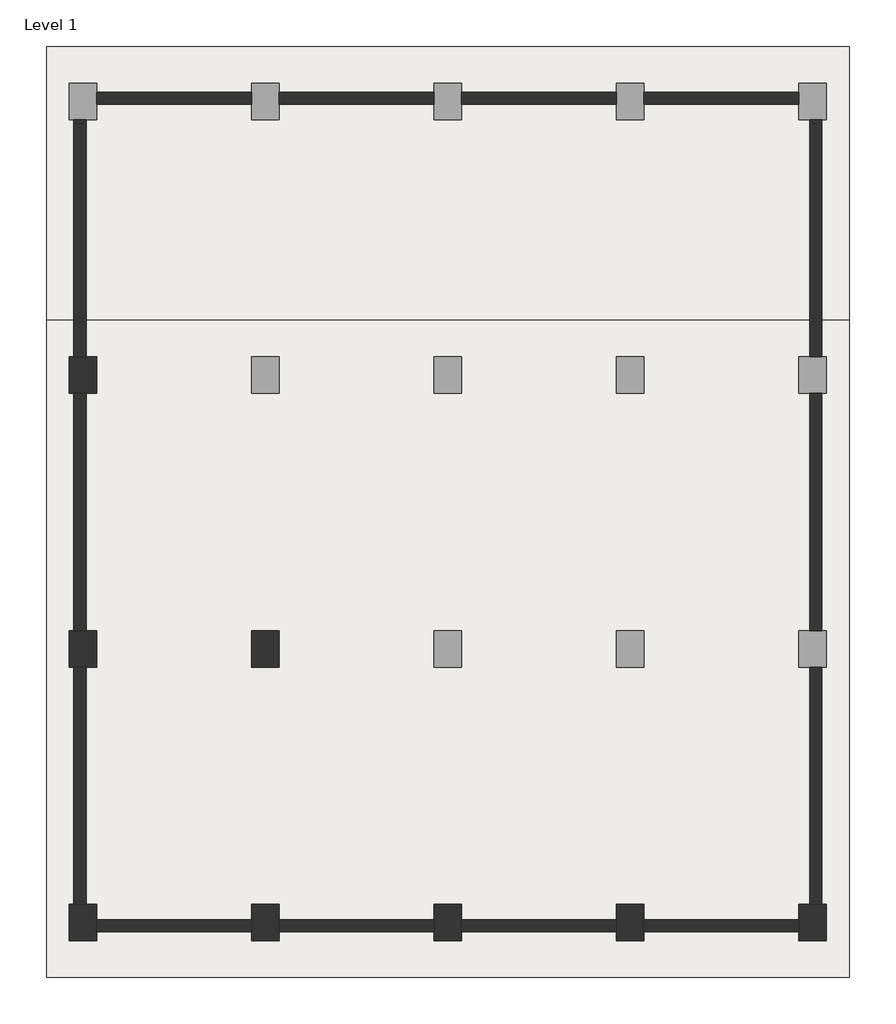
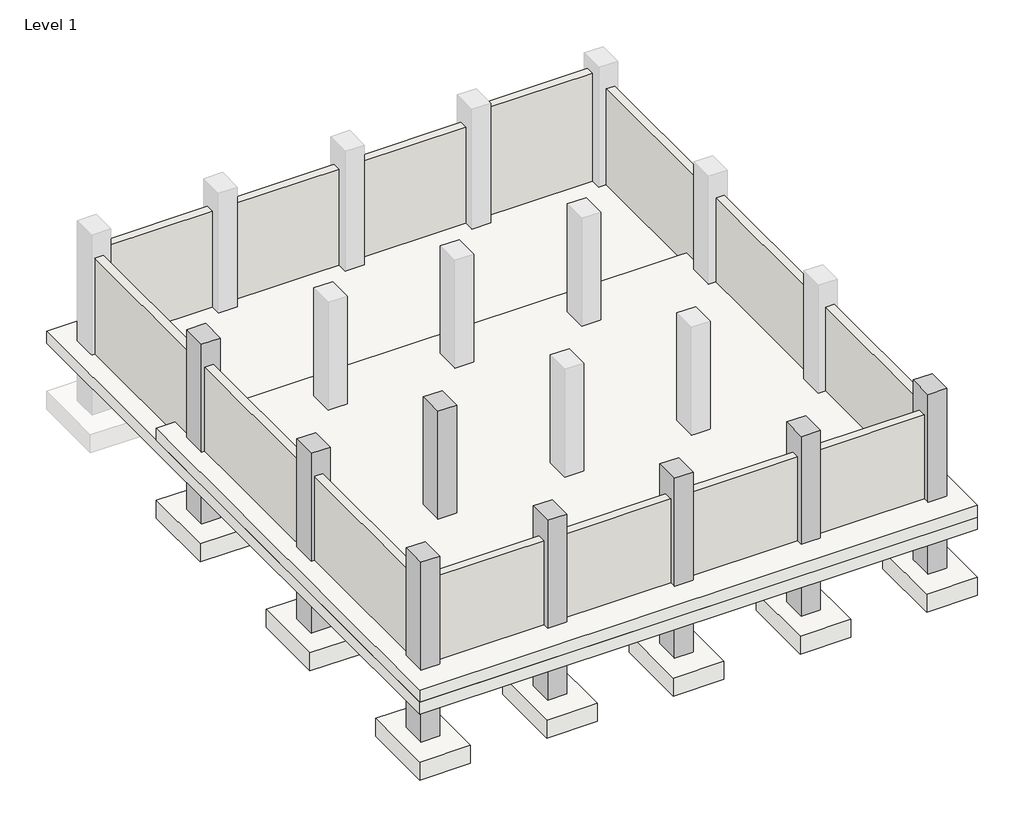
# One storey, part 1 of 2: 14 walls, 12 beams, 9 slabs, 8 columns, 2 roofs.
"""IFC4 building model written with IfcOpenShell, lengths in millimetres."""

from ifc_helpers import new_model, si_unit, frame, origin, origin_with_axes, place, context, project, spatial, polyline, outline, extrude, faceted_brep, transform, mapped, element, save
from components import slab_5ba74754

model = new_model("IFC4")

# Units and contexts
model_context = context("Model", 3, world=origin())
ifc_project = project(units=[si_unit("LENGTHUNIT", "METRE", prefix="MILLI")], contexts=[model_context])

# Site, building, storey
site = spatial("IfcSite", under=ifc_project)
building = spatial("IfcBuilding", under=site)
storey = spatial("IfcBuildingStorey", under=building, Name="Level 1", Elevation=0.0)

# Beams
placement = place(None, origin())
element("IfcBeam", 1, ObjectType="Concrete-Rectangular Beam : 12 x 24", at=placement, inside=storey, context=model_context, shape_type="SweptSolid", body=[
    extrude(outline(polyline([(-21772.1183349, 4163.0075069), (-21467.3183349, 4163.0075069), (-21467.3183349, 200.6075069), (-21772.1183349, 200.6075069), (-21772.1183349, 4163.0075069)])), frame((0.0, 0.0, -609.6), z_axis=(0.0, 0.0, 1.0), x_axis=(1.0, 0.0, 0.0)), (0.0, 0.0, 1.0), 304.8),
])
element("IfcBeam", 2, ObjectType="Concrete-Rectangular Beam : 12 x 24", at=placement, inside=storey, context=model_context, shape_type="SweptSolid", body=[
    extrude(outline(polyline([(-21772.1183349, 8735.0075069), (-21467.3183349, 8735.0075069), (-21467.3183349, 4772.6075069), (-21772.1183349, 4772.6075069), (-21772.1183349, 8735.0075069)])), frame((0.0, 0.0, -609.6), z_axis=(0.0, 0.0, 1.0), x_axis=(1.0, 0.0, 0.0)), (0.0, 0.0, 1.0), 304.8),
])
element("IfcBeam", 3, ObjectType="Concrete-Rectangular Beam : 12 x 24", at=placement, inside=storey, context=model_context, shape_type="SweptSolid", body=[
    extrude(outline(polyline([(-21772.1183349, 13307.0075069), (-21467.3183349, 13307.0075069), (-21467.3183349, 9344.6075069), (-21772.1183349, 9344.6075069), (-21772.1183349, 13307.0075069)])), frame((0.0, 0.0, -609.6), z_axis=(0.0, 0.0, 1.0), x_axis=(1.0, 0.0, 0.0)), (0.0, 0.0, 1.0), 304.8),
])
element("IfcBeam", 4, ObjectType="Concrete-Rectangular Beam : 12 x 24", at=placement, inside=storey, context=model_context, shape_type="SweptSolid", body=[
    extrude(outline(polyline([(-18724.1183349, 4163.0075069), (-18419.3183349, 4163.0075069), (-18419.3183349, 200.6075069), (-18724.1183349, 200.6075069), (-18724.1183349, 4163.0075069)])), frame((0.0, 0.0, -609.6), z_axis=(0.0, 0.0, 1.0), x_axis=(1.0, 0.0, 0.0)), (0.0, 0.0, 1.0), 304.8),
])
element("IfcBeam", 5, ObjectType="Concrete-Rectangular Beam : 12 x 24", at=placement, inside=storey, context=model_context, shape_type="SweptSolid", body=[
    extrude(outline(polyline([(-18724.1183349, 8735.0075069), (-18419.3183349, 8735.0075069), (-18419.3183349, 4772.6075069), (-18724.1183349, 4772.6075069), (-18724.1183349, 8735.0075069)])), frame((0.0, 0.0, -609.6), z_axis=(0.0, 0.0, 1.0), x_axis=(1.0, 0.0, 0.0)), (0.0, 0.0, 1.0), 304.8),
])
element("IfcBeam", 6, ObjectType="Concrete-Rectangular Beam : 12 x 24", at=placement, inside=storey, context=model_context, shape_type="SweptSolid", body=[
    extrude(outline(polyline([(-21391.1183349, 8887.4075069), (-21391.1183349, 9192.2075069), (-18800.3183349, 9192.2075069), (-18800.3183349, 8887.4075069), (-21391.1183349, 8887.4075069)])), frame((0.0, 0.0, -609.6), z_axis=(0.0, 0.0, 1.0), x_axis=(1.0, 0.0, 0.0)), (0.0, 0.0, 1.0), 304.8),
])
element("IfcBeam", 7, ObjectType="Concrete-Rectangular Beam : 12 x 24", at=placement, inside=storey, context=model_context, shape_type="SweptSolid", body=[
    extrude(outline(polyline([(-21391.1183349, 4315.4075069), (-21391.1183349, 4620.2075069), (-18800.3183349, 4620.2075069), (-18800.3183349, 4315.4075069), (-21391.1183349, 4315.4075069)])), frame((0.0, 0.0, -609.6), z_axis=(0.0, 0.0, 1.0), x_axis=(1.0, 0.0, 0.0)), (0.0, 0.0, 1.0), 304.8),
])
element("IfcBeam", 8, ObjectType="Concrete-Rectangular Beam : 12 x 24", at=placement, inside=storey, context=model_context, shape_type="SweptSolid", body=[
    extrude(outline(polyline([(-18343.1183349, 4315.4075069), (-18343.1183349, 4620.2075069), (-15752.3183349, 4620.2075069), (-15752.3183349, 4315.4075069), (-18343.1183349, 4315.4075069)])), frame((0.0, 0.0, -609.6), z_axis=(0.0, 0.0, 1.0), x_axis=(1.0, 0.0, 0.0)), (0.0, 0.0, 1.0), 304.8),
])
element("IfcBeam", 9, ObjectType="Concrete-Rectangular Beam : 12 x 24", at=placement, inside=storey, context=model_context, shape_type="SweptSolid", body=[
    extrude(outline(polyline([(-21391.1183349, -256.5924931), (-21391.1183349, 48.2075069), (-18800.3183349, 48.2075069), (-18800.3183349, -256.5924931), (-21391.1183349, -256.5924931)])), frame((0.0, 0.0, -609.6), z_axis=(0.0, 0.0, 1.0), x_axis=(1.0, 0.0, 0.0)), (0.0, 0.0, 1.0), 304.8),
])
element("IfcBeam", 10, ObjectType="Concrete-Rectangular Beam : 12 x 24", at=placement, inside=storey, context=model_context, shape_type="SweptSolid", body=[
    extrude(outline(polyline([(-18343.1183349, -256.5924931), (-18343.1183349, 48.2075069), (-15752.3183349, 48.2075069), (-15752.3183349, -256.5924931), (-18343.1183349, -256.5924931)])), frame((0.0, 0.0, -609.6), z_axis=(0.0, 0.0, 1.0), x_axis=(1.0, 0.0, 0.0)), (0.0, 0.0, 1.0), 304.8),
])
element("IfcBeam", 11, ObjectType="Concrete-Rectangular Beam : 12 x 24", at=placement, inside=storey, context=model_context, shape_type="SweptSolid", body=[
    extrude(outline(polyline([(-15295.1183349, -256.5924931), (-15295.1183349, 48.2075069), (-12704.3183349, 48.2075069), (-12704.3183349, -256.5924931), (-15295.1183349, -256.5924931)])), frame((0.0, 0.0, -609.6), z_axis=(0.0, 0.0, 1.0), x_axis=(1.0, 0.0, 0.0)), (0.0, 0.0, 1.0), 304.8),
])
element("IfcBeam", 12, ObjectType="Concrete-Rectangular Beam : 12 x 24", at=placement, inside=storey, context=model_context, shape_type="SweptSolid", body=[
    extrude(outline(polyline([(-12247.1183349, -256.5924931), (-12247.1183349, 48.2075069), (-9656.3183349, 48.2075069), (-9656.3183349, -256.5924931), (-12247.1183349, -256.5924931)])), frame((0.0, 0.0, -609.6), z_axis=(0.0, 0.0, 1.0), x_axis=(1.0, 0.0, 0.0)), (0.0, 0.0, 1.0), 304.8),
])

# Columns
element("IfcColumn", 13, ObjectType="Concrete-Rectangular-Column : 18 x 24", at=placement, inside=storey, context=model_context, shape_type="Brep", body=[
    faceted_brep([(-21391.1183349, 9344.6075069, -1524.0), (-21391.1183349, 8735.0075069, -1524.0), (-21848.3183349, 8735.0075069, -1524.0), (-21848.3183349, 9344.6075069, -1524.0), (-21391.1183349, 8735.0075069, -304.8), (-21391.1183349, 9344.6075069, -304.8), (-21848.3183349, 9344.6075069, -304.8), (-21848.3183349, 8735.0075069, -304.8)], [[[0, 1, 2, 3]], [[4, 5, 6, 7]], [[1, 0, 5, 4]], [[2, 1, 4, 7]], [[3, 2, 7, 6]], [[0, 3, 6, 5]]]),
    faceted_brep([(-21391.1183349, 9344.6075069, 3048.0), (-21391.1183349, 8735.0075069, 3048.0), (-21391.1183349, 8735.0075069, 0.0), (-21391.1183349, 9344.6075069, 0.0), (-21848.3183349, 8735.0075069, 3048.0), (-21848.3183349, 8735.0075069, 0.0), (-21772.1183349, 8735.0075069, 0.0), (-21568.9183349, 8735.0075069, 0.0), (-21848.3183349, 9344.6075069, 3048.0), (-21848.3183349, 9344.6075069, 0.0), (-21568.9183349, 9344.6075069, 0.0), (-21772.1183349, 9344.6075069, 0.0)], [[[0, 1, 2, 3]], [[1, 4, 5, 6, 7, 2]], [[4, 8, 9, 5]], [[8, 0, 3, 10, 11, 9]], [[1, 0, 8, 4]], [[3, 2, 7, 6, 5, 9, 11, 10]]]),
])
element("IfcColumn", 14, ObjectType="Concrete-Rectangular-Column : 18 x 24", at=placement, inside=storey, context=model_context, shape_type="Brep", body=[
    faceted_brep([(-21391.1183349, 4772.6075069, -1524.0), (-21391.1183349, 4163.0075069, -1524.0), (-21848.3183349, 4163.0075069, -1524.0), (-21848.3183349, 4772.6075069, -1524.0), (-21391.1183349, 4163.0075069, -304.8), (-21391.1183349, 4772.6075069, -304.8), (-21848.3183349, 4772.6075069, -304.8), (-21848.3183349, 4163.0075069, -304.8)], [[[0, 1, 2, 3]], [[4, 5, 6, 7]], [[1, 0, 5, 4]], [[2, 1, 4, 7]], [[3, 2, 7, 6]], [[0, 3, 6, 5]]]),
    faceted_brep([(-21391.1183349, 4772.6075069, 3048.0), (-21391.1183349, 4163.0075069, 3048.0), (-21391.1183349, 4163.0075069, 0.0), (-21391.1183349, 4772.6075069, 0.0), (-21848.3183349, 4163.0075069, 3048.0), (-21848.3183349, 4163.0075069, 0.0), (-21772.1183349, 4163.0075069, 0.0), (-21568.9183349, 4163.0075069, 0.0), (-21848.3183349, 4772.6075069, 3048.0), (-21848.3183349, 4772.6075069, 0.0), (-21568.9183349, 4772.6075069, 0.0), (-21772.1183349, 4772.6075069, 0.0)], [[[0, 1, 2, 3]], [[1, 4, 5, 6, 7, 2]], [[4, 8, 9, 5]], [[8, 0, 3, 10, 11, 9]], [[1, 0, 8, 4]], [[3, 2, 7, 6, 5, 9, 11, 10]]]),
])
element("IfcColumn", 15, ObjectType="Concrete-Rectangular-Column : 18 x 24", at=placement, inside=storey, context=model_context, shape_type="Brep", body=[
    faceted_brep([(-21391.1183349, 200.6075069, -1524.0), (-21391.1183349, -408.9924931, -1524.0), (-21848.3183349, -408.9924931, -1524.0), (-21848.3183349, 200.6075069, -1524.0), (-21391.1183349, -408.9924931, -304.8), (-21391.1183349, 200.6075069, -304.8), (-21848.3183349, 200.6075069, -304.8), (-21848.3183349, -408.9924931, -304.8)], [[[0, 1, 2, 3]], [[4, 5, 6, 7]], [[1, 0, 5, 4]], [[2, 1, 4, 7]], [[3, 2, 7, 6]], [[0, 3, 6, 5]]]),
    faceted_brep([(-21391.1183349, 200.6075069, 3048.0), (-21391.1183349, -408.9924931, 3048.0), (-21391.1183349, -408.9924931, 0.0), (-21391.1183349, -256.5924931, 0.0), (-21391.1183349, -53.3924931, 0.0), (-21391.1183349, 200.6075069, 0.0), (-21848.3183349, -408.9924931, 3048.0), (-21848.3183349, -408.9924931, 0.0), (-21848.3183349, 200.6075069, 3048.0), (-21848.3183349, 200.6075069, 0.0), (-21568.9183349, 200.6075069, 0.0), (-21772.1183349, 200.6075069, 0.0)], [[[0, 1, 2, 3, 4, 5]], [[1, 6, 7, 2]], [[6, 8, 9, 7]], [[8, 0, 5, 10, 11, 9]], [[1, 0, 8, 6]], [[5, 4, 3, 2, 7, 9, 11, 10]]]),
])
element("IfcColumn", 16, ObjectType="Concrete-Rectangular-Column : 18 x 24", at=placement, inside=storey, context=model_context, shape_type="SweptSolid", body=[
    extrude(outline(polyline([(-18343.1183349, 4772.6075069), (-18343.1183349, 4163.0075069), (-18800.3183349, 4163.0075069), (-18800.3183349, 4772.6075069), (-18343.1183349, 4772.6075069)])), frame((0.0, 0.0, -1524.0), z_axis=(0.0, 0.0, 1.0), x_axis=(1.0, 0.0, 0.0)), (0.0, 0.0, 1.0), 1219.2),
    extrude(outline(polyline([(-18343.1183349, 4772.6075069), (-18343.1183349, 4163.0075069), (-18800.3183349, 4163.0075069), (-18800.3183349, 4772.6075069), (-18343.1183349, 4772.6075069)])), origin_with_axes(), (0.0, 0.0, 1.0), 3048.0),
])
element("IfcColumn", 17, ObjectType="Concrete-Rectangular-Column : 18 x 24", at=placement, inside=storey, context=model_context, shape_type="Brep", body=[
    faceted_brep([(-18343.1183349, 200.6075069, -1524.0), (-18343.1183349, -408.9924931, -1524.0), (-18800.3183349, -408.9924931, -1524.0), (-18800.3183349, 200.6075069, -1524.0), (-18343.1183349, -408.9924931, -304.8), (-18343.1183349, 200.6075069, -304.8), (-18800.3183349, 200.6075069, -304.8), (-18800.3183349, -408.9924931, -304.8)], [[[0, 1, 2, 3]], [[4, 5, 6, 7]], [[1, 0, 5, 4]], [[2, 1, 4, 7]], [[3, 2, 7, 6]], [[0, 3, 6, 5]]]),
    faceted_brep([(-18343.1183349, 200.6075069, 3048.0), (-18343.1183349, -408.9924931, 3048.0), (-18343.1183349, -408.9924931, 0.0), (-18343.1183349, -256.5924931, 0.0), (-18343.1183349, -53.3924931, 0.0), (-18343.1183349, 200.6075069, 0.0), (-18800.3183349, -408.9924931, 3048.0), (-18800.3183349, -408.9924931, 0.0), (-18800.3183349, 200.6075069, 3048.0), (-18800.3183349, 200.6075069, 0.0), (-18800.3183349, -53.3924931, 0.0), (-18800.3183349, -256.5924931, 0.0)], [[[0, 1, 2, 3, 4, 5]], [[1, 6, 7, 2]], [[6, 8, 9, 10, 11, 7]], [[8, 0, 5, 9]], [[1, 0, 8, 6]], [[5, 4, 3, 2, 7, 11, 10, 9]]]),
])
element("IfcColumn", 18, ObjectType="Concrete-Rectangular-Column : 18 x 24", at=placement, inside=storey, context=model_context, shape_type="Brep", body=[
    faceted_brep([(-15295.1183349, 200.6075069, -1524.0), (-15295.1183349, -408.9924931, -1524.0), (-15752.3183349, -408.9924931, -1524.0), (-15752.3183349, 200.6075069, -1524.0), (-15295.1183349, -408.9924931, -304.8), (-15295.1183349, 200.6075069, -304.8), (-15752.3183349, 200.6075069, -304.8), (-15752.3183349, -408.9924931, -304.8)], [[[0, 1, 2, 3]], [[4, 5, 6, 7]], [[1, 0, 5, 4]], [[2, 1, 4, 7]], [[3, 2, 7, 6]], [[0, 3, 6, 5]]]),
    faceted_brep([(-15295.1183349, 200.6075069, 3048.0), (-15295.1183349, -408.9924931, 3048.0), (-15295.1183349, -408.9924931, 0.0), (-15295.1183349, -256.5924931, 0.0), (-15295.1183349, -53.3924931, 0.0), (-15295.1183349, 200.6075069, 0.0), (-15752.3183349, -408.9924931, 3048.0), (-15752.3183349, -408.9924931, 0.0), (-15752.3183349, 200.6075069, 3048.0), (-15752.3183349, 200.6075069, 0.0), (-15752.3183349, -53.3924931, 0.0), (-15752.3183349, -256.5924931, 0.0)], [[[0, 1, 2, 3, 4, 5]], [[1, 6, 7, 2]], [[6, 8, 9, 10, 11, 7]], [[8, 0, 5, 9]], [[1, 0, 8, 6]], [[5, 4, 3, 2, 7, 11, 10, 9]]]),
])
element("IfcColumn", 19, ObjectType="Concrete-Rectangular-Column : 18 x 24", at=placement, inside=storey, context=model_context, shape_type="Brep", body=[
    faceted_brep([(-12247.1183349, 200.6075069, -1524.0), (-12247.1183349, -408.9924931, -1524.0), (-12704.3183349, -408.9924931, -1524.0), (-12704.3183349, 200.6075069, -1524.0), (-12247.1183349, -408.9924931, -304.8), (-12247.1183349, 200.6075069, -304.8), (-12704.3183349, 200.6075069, -304.8), (-12704.3183349, -408.9924931, -304.8)], [[[0, 1, 2, 3]], [[4, 5, 6, 7]], [[1, 0, 5, 4]], [[2, 1, 4, 7]], [[3, 2, 7, 6]], [[0, 3, 6, 5]]]),
    faceted_brep([(-12247.1183349, 200.6075069, 3048.0), (-12247.1183349, -408.9924931, 3048.0), (-12247.1183349, -408.9924931, 0.0), (-12247.1183349, -256.5924931, 0.0), (-12247.1183349, -53.3924931, 0.0), (-12247.1183349, 200.6075069, 0.0), (-12704.3183349, -408.9924931, 3048.0), (-12704.3183349, -408.9924931, 0.0), (-12704.3183349, 200.6075069, 3048.0), (-12704.3183349, 200.6075069, 0.0), (-12704.3183349, -53.3924931, 0.0), (-12704.3183349, -256.5924931, 0.0)], [[[0, 1, 2, 3, 4, 5]], [[1, 6, 7, 2]], [[6, 8, 9, 10, 11, 7]], [[8, 0, 5, 9]], [[1, 0, 8, 6]], [[5, 4, 3, 2, 7, 11, 10, 9]]]),
])
element("IfcColumn", 20, ObjectType="Concrete-Rectangular-Column : 18 x 24", at=placement, inside=storey, context=model_context, shape_type="Brep", body=[
    faceted_brep([(-9199.1183349, 200.6075069, -1524.0), (-9199.1183349, -408.9924931, -1524.0), (-9656.3183349, -408.9924931, -1524.0), (-9656.3183349, 200.6075069, -1524.0), (-9199.1183349, -408.9924931, -304.8), (-9199.1183349, 200.6075069, -304.8), (-9656.3183349, 200.6075069, -304.8), (-9656.3183349, -408.9924931, -304.8)], [[[0, 1, 2, 3]], [[4, 5, 6, 7]], [[1, 0, 5, 4]], [[2, 1, 4, 7]], [[3, 2, 7, 6]], [[0, 3, 6, 5]]]),
    faceted_brep([(-9199.1183349, 200.6075069, 3048.0), (-9199.1183349, -408.9924931, 3048.0), (-9199.1183349, -408.9924931, 0.0), (-9199.1183349, 200.6075069, 0.0), (-9656.3183349, -408.9924931, 3048.0), (-9656.3183349, -408.9924931, 0.0), (-9656.3183349, 200.6075069, 3048.0), (-9656.3183349, 200.6075069, 0.0), (-9656.3183349, -53.3924931, 0.0), (-9656.3183349, -256.5924931, 0.0), (-9275.3183349, 200.6075069, 0.0), (-9478.5183349, 200.6075069, 0.0)], [[[0, 1, 2, 3]], [[1, 4, 5, 2]], [[4, 6, 7, 8, 9, 5]], [[6, 0, 3, 10, 11, 7]], [[1, 0, 6, 4]], [[3, 2, 5, 9, 8, 7, 11, 10]]]),
])

# Roofs
element("IfcRoof", 21, ObjectType="Generic - 12\"", at=placement, inside=storey, context=model_context, shape_type="SweptSolid", body=[
    extrude(outline(polyline([(-22229.3183349, 9954.2075069), (-8818.1183349, 9954.2075069), (-8818.1183349, -1018.5924931), (-22229.3183349, -1018.5924931), (-22229.3183349, 9954.2075069)])), origin_with_axes(), (0.0, 0.0, 1.0), 304.8),
])
element("IfcRoof", 22, ObjectType="Generic - 12\"", at=placement, inside=storey, context=model_context, shape_type="SweptSolid", body=[
    extrude(outline(polyline([(-22229.3183349, 9954.2075069), (-8818.1183349, 9954.2075069), (-8818.1183349, -1018.5924931), (-22229.3183349, -1018.5924931), (-22229.3183349, 9954.2075069)])), origin_with_axes(), (0.0, 0.0, 1.0), 304.8),
])

# Slabs
slab_shape = slab_5ba74754(model_context)
element("IfcSlab", 23, ObjectType="Footing-Rectangular : 72\" x 48\" x 18\"", at=placement, inside=storey, context=model_context, shape_type="MappedRepresentation", body=[
    mapped(slab_shape, transform((-21619.7183349, 9039.8075069, -1524.0), x_axis=(1.0, 0.0, 0.0), y_axis=(0.0, 1.0, 0.0), z_axis=(0.0, 0.0, 1.0))),
])
element("IfcSlab", 24, ObjectType="Footing-Rectangular : 72\" x 48\" x 18\"", at=placement, inside=storey, context=model_context, shape_type="MappedRepresentation", body=[
    mapped(slab_shape, transform((-21619.7183349, 4467.8075069, -1524.0), x_axis=(1.0, 0.0, 0.0), y_axis=(0.0, 1.0, 0.0), z_axis=(0.0, 0.0, 1.0))),
])
element("IfcSlab", 25, ObjectType="Footing-Rectangular : 72\" x 48\" x 18\"", at=placement, inside=storey, context=model_context, shape_type="MappedRepresentation", body=[
    mapped(slab_shape, transform((-21619.7183349, -104.1924931, -1524.0), x_axis=(1.0, 0.0, 0.0), y_axis=(0.0, 1.0, 0.0), z_axis=(0.0, 0.0, 1.0))),
])
element("IfcSlab", 26, ObjectType="Footing-Rectangular : 72\" x 48\" x 18\"", at=placement, inside=storey, context=model_context, shape_type="MappedRepresentation", body=[
    mapped(slab_shape, transform((-18571.7183349, 4467.8075069, -1524.0), x_axis=(1.0, 0.0, 0.0), y_axis=(0.0, 1.0, 0.0), z_axis=(0.0, 0.0, 1.0))),
])
element("IfcSlab", 27, ObjectType="Footing-Rectangular : 72\" x 48\" x 18\"", at=placement, inside=storey, context=model_context, shape_type="MappedRepresentation", body=[
    mapped(slab_shape, transform((-18571.7183349, -104.1924931, -1524.0), x_axis=(1.0, 0.0, 0.0), y_axis=(0.0, 1.0, 0.0), z_axis=(0.0, 0.0, 1.0))),
])
element("IfcSlab", 28, ObjectType="Footing-Rectangular : 72\" x 48\" x 18\"", at=placement, inside=storey, context=model_context, shape_type="MappedRepresentation", body=[
    mapped(slab_shape, transform((-15523.7183349, -104.1924931, -1524.0), x_axis=(1.0, 0.0, 0.0), y_axis=(0.0, 1.0, 0.0), z_axis=(0.0, 0.0, 1.0))),
])
element("IfcSlab", 29, ObjectType="Footing-Rectangular : 72\" x 48\" x 18\"", at=placement, inside=storey, context=model_context, shape_type="MappedRepresentation", body=[
    mapped(slab_shape, transform((-12475.7183349, -104.1924931, -1524.0), x_axis=(1.0, 0.0, 0.0), y_axis=(0.0, 1.0, 0.0), z_axis=(0.0, 0.0, 1.0))),
])
element("IfcSlab", 30, ObjectType="Footing-Rectangular : 72\" x 48\" x 18\"", at=placement, inside=storey, context=model_context, shape_type="MappedRepresentation", body=[
    mapped(slab_shape, transform((-9427.7183349, -104.1924931, -1524.0), x_axis=(1.0, 0.0, 0.0), y_axis=(0.0, 1.0, 0.0), z_axis=(0.0, 0.0, 1.0))),
])
element("IfcSlab", 31, ObjectType="Generic - 12\"", at=placement, inside=storey, context=model_context, shape_type="SweptSolid", body=[
    extrude(outline(polyline([(-8818.1183349, 14526.2075069), (-8818.1183349, -1018.5924931), (-22229.3183349, -1018.5924931), (-22229.3183349, 14526.2075069), (-8818.1183349, 14526.2075069)])), frame((0.0, 0.0, -304.8), z_axis=(0.0, 0.0, 1.0), x_axis=(1.0, 0.0, 0.0)), (0.0, 0.0, 1.0), 304.8),
])

# Walls
element("IfcWall", 32, ObjectType="Generic - 8\"", at=placement, inside=storey, context=model_context, shape_type="SweptSolid", body=[
    extrude(outline(polyline([(-21772.1183349, 9344.6075069), (-21772.1183349, 13307.0075069), (-21568.9183349, 13307.0075069), (-21568.9183349, 9344.6075069), (-21772.1183349, 9344.6075069)])), origin_with_axes(), (0.0, 0.0, 1.0), 2438.4),
])
element("IfcWall", 33, ObjectType="Generic - 8\"", at=placement, inside=storey, context=model_context, shape_type="SweptSolid", body=[
    extrude(outline(polyline([(-21772.1183349, 4772.6075069), (-21772.1183349, 8735.0075069), (-21568.9183349, 8735.0075069), (-21568.9183349, 4772.6075069), (-21772.1183349, 4772.6075069)])), origin_with_axes(), (0.0, 0.0, 1.0), 2438.4),
])
element("IfcWall", 34, ObjectType="Generic - 8\"", at=placement, inside=storey, context=model_context, shape_type="SweptSolid", body=[
    extrude(outline(polyline([(-21772.1183349, 200.6075069), (-21772.1183349, 4163.0075069), (-21568.9183349, 4163.0075069), (-21568.9183349, 200.6075069), (-21772.1183349, 200.6075069)])), origin_with_axes(), (0.0, 0.0, 1.0), 2438.4),
])
element("IfcWall", 35, ObjectType="Generic - 8\"", at=placement, inside=storey, context=model_context, shape_type="SweptSolid", body=[
    extrude(outline(polyline([(-18800.3183349, -256.5924931), (-21391.1183349, -256.5924931), (-21391.1183349, -53.3924931), (-18800.3183349, -53.3924931), (-18800.3183349, -256.5924931)])), origin_with_axes(), (0.0, 0.0, 1.0), 2438.4),
])
element("IfcWall", 36, ObjectType="Generic - 8\"", at=placement, inside=storey, context=model_context, shape_type="SweptSolid", body=[
    extrude(outline(polyline([(-15752.3183349, -256.5924931), (-18343.1183349, -256.5924931), (-18343.1183349, -53.3924931), (-15752.3183349, -53.3924931), (-15752.3183349, -256.5924931)])), origin_with_axes(), (0.0, 0.0, 1.0), 2438.4),
])
element("IfcWall", 37, ObjectType="Generic - 8\"", at=placement, inside=storey, context=model_context, shape_type="SweptSolid", body=[
    extrude(outline(polyline([(-12704.3183349, -256.5924931), (-15295.1183349, -256.5924931), (-15295.1183349, -53.3924931), (-12704.3183349, -53.3924931), (-12704.3183349, -256.5924931)])), origin_with_axes(), (0.0, 0.0, 1.0), 2438.4),
])
element("IfcWall", 38, ObjectType="Generic - 8\"", at=placement, inside=storey, context=model_context, shape_type="SweptSolid", body=[
    extrude(outline(polyline([(-9656.3183349, -256.5924931), (-12247.1183349, -256.5924931), (-12247.1183349, -53.3924931), (-9656.3183349, -53.3924931), (-9656.3183349, -256.5924931)])), origin_with_axes(), (0.0, 0.0, 1.0), 2438.4),
])
element("IfcWall", 39, ObjectType="Generic - 8\"", at=placement, inside=storey, context=model_context, shape_type="SweptSolid", body=[
    extrude(outline(polyline([(-9478.5183349, 9344.6075069), (-9478.5183349, 13307.0075069), (-9275.3183349, 13307.0075069), (-9275.3183349, 9344.6075069), (-9478.5183349, 9344.6075069)])), origin_with_axes(), (0.0, 0.0, 1.0), 2438.4),
])
element("IfcWall", 40, ObjectType="Generic - 8\"", at=placement, inside=storey, context=model_context, shape_type="SweptSolid", body=[
    extrude(outline(polyline([(-9478.5183349, 4772.6075069), (-9478.5183349, 8735.0075069), (-9275.3183349, 8735.0075069), (-9275.3183349, 4772.6075069), (-9478.5183349, 4772.6075069)])), origin_with_axes(), (0.0, 0.0, 1.0), 2438.4),
])
element("IfcWall", 41, ObjectType="Generic - 8\"", at=placement, inside=storey, context=model_context, shape_type="SweptSolid", body=[
    extrude(outline(polyline([(-9478.5183349, 200.6075069), (-9478.5183349, 4163.0075069), (-9275.3183349, 4163.0075069), (-9275.3183349, 200.6075069), (-9478.5183349, 200.6075069)])), origin_with_axes(), (0.0, 0.0, 1.0), 2438.4),
])
element("IfcWall", 42, ObjectType="Generic - 8\"", at=placement, inside=storey, context=model_context, shape_type="SweptSolid", body=[
    extrude(outline(polyline([(-18800.3183349, 13561.0075069), (-21391.1183349, 13561.0075069), (-21391.1183349, 13764.2075069), (-18800.3183349, 13764.2075069), (-18800.3183349, 13561.0075069)])), origin_with_axes(), (0.0, 0.0, 1.0), 2438.4),
])
element("IfcWall", 43, ObjectType="Generic - 8\"", at=placement, inside=storey, context=model_context, shape_type="SweptSolid", body=[
    extrude(outline(polyline([(-15752.3183349, 13561.0075069), (-18343.1183349, 13561.0075069), (-18343.1183349, 13764.2075069), (-15752.3183349, 13764.2075069), (-15752.3183349, 13561.0075069)])), origin_with_axes(), (0.0, 0.0, 1.0), 2438.4),
])
element("IfcWall", 44, ObjectType="Generic - 8\"", at=placement, inside=storey, context=model_context, shape_type="SweptSolid", body=[
    extrude(outline(polyline([(-12704.3183349, 13561.0075069), (-15295.1183349, 13561.0075069), (-15295.1183349, 13764.2075069), (-12704.3183349, 13764.2075069), (-12704.3183349, 13561.0075069)])), origin_with_axes(), (0.0, 0.0, 1.0), 2438.4),
])
element("IfcWall", 45, ObjectType="Generic - 8\"", at=placement, inside=storey, context=model_context, shape_type="Brep", body=[
    faceted_brep([(-12247.1183349, 13561.0075069, 0.0), (-9656.3183349, 13561.0075069, 0.0), (-9656.3183349, 13561.0075069, 2438.4), (-9656.3183349, 13561.0075069, 2743.2), (-12247.1183349, 13561.0075069, 2743.2), (-12247.1183349, 13561.0075069, 2438.4), (-12247.1183349, 13764.2075069, 0.0), (-12247.1183349, 13764.2075069, 2743.2), (-9656.3183349, 13764.2075069, 2743.2), (-9656.3183349, 13764.2075069, 0.0)], [[[0, 1, 2, 3, 4, 5]], [[6, 7, 8, 9]], [[1, 0, 6, 9]], [[3, 2, 1, 9, 8]], [[4, 3, 8, 7]], [[0, 5, 4, 7, 6]]]),
])

save(model, "model.ifc")

# Revit data of these elements
# Grids (mm)
#   "1": line (-21619.718, 15603.605) -> (-21619.718, -4395.845)
#   "2": line (-18571.718, 15603.605) -> (-18571.718, -4395.845)
#   "3": line (-15523.718, 15603.605) -> (-15523.718, -4395.845)
#   "4": line (-12475.718, 15603.605) -> (-12475.718, -4395.845)
#   "5": line (-9427.718, 15603.605) -> (-9427.718, -4395.845)
#   "7": line (-5253.178, 9039.808) -> (-25779.985, 9039.808)
#   "8": line (-5253.178, 4467.808) -> (-25779.985, 4467.808)
#   "9": line (-5253.178, -104.192) -> (-25779.985, -104.192)
#   "6": line (-5253.178, 13611.808) -> (-25779.985, 13611.808)
# Type "Concrete-Rectangular Beam : 12 x 24"
#   Assembly Code = "B10"
#   Length [instance default] = 5' - 0"
#   b = 1' - 0"
#   h = 2' - 0"
#   Structural Material [instance default] = Concrete, Cast-in-Place gray
# Type "Concrete-Rectangular-Column : 18 x 24"
#   Assembly Code = "B10"
#   b = 1' - 6"
#   h = 2' - 0"
#   Structural Material [instance default] = Concrete, Cast-in-Place gray
# Type "Generic - 12\""
#   Assembly Code = "B1020"
#   Layers, outside or top first: 1' - 0" no material (function 1)
# Type "Footing-Rectangular : 72\" x 48\" x 18\""
#   Assembly Code = "A1010100"
#   Width = 4' - 0"
#   Length = 6' - 0"
#   Foundation Thickness = 1' - 6"
#   Structural Material [instance default] = Concrete, Cast-in-Place gray
# Type "Generic - 12\""
#   Assembly Code = "B1010"
#   Function = 0
#   Layers, outside or top first: 1' - 0" no material (function 1)
# Type "Generic - 8\""
#   Assembly Code = "B2010"
#   Layers, outside or top first: 0' - 8" no material (function 1)
# Elements 1, 2, 3, 4, 5, 6, 7, 8, 9, 10, 11, 12 (IfcBeam, "Concrete-Rectangular Beam : 12 x 24")
#   Structural Material = Concrete, Cast-in-Place gray
#   Phase Created = New Construction
#   Materials on its faces: "Concrete, Cast-in-Place gray"
# Elements 13, 14, 15, 16, 17, 18, 19, 20 (IfcColumn, "Concrete-Rectangular-Column : 18 x 24")
#   Structural Material = Concrete, Cast-in-Place gray
#   Phase Created = New Construction
#   Materials on its faces: "Concrete, Cast-in-Place gray"
# Elements 21, 22 (IfcRoof, "Generic - 12\"")
#   built-in parameter 1001705 = 1 (stored number, unit not read)
#   built-in parameter 1001710 = 33615
#   Phase Created = New Construction
#   Materials on its faces: "Default Roof"
# Elements 23, 24, 25, 26, 27, 28, 29, 30 (IfcSlab, "Footing-Rectangular : 72\" x 48\" x 18\"")
#   Structural Material = Concrete, Cast-in-Place gray
#   Phase Created = New Construction
#   Materials on its faces: "Concrete, Cast-in-Place gray"
# Element 31 (IfcSlab, "Generic - 12\"")
#   Height Offset From Level = 0' - 0"
#   built-in parameter 1001954 = 1
#   Phase Created = New Construction
#   Materials on its faces: "Default Floor"
# Elements 32, 33, 34, 35, 36, 37, 38, 39, 40, 41, 42, 43, 44 (IfcWall, "Generic - 8\"")
#   Top Offset = -2' - 0"
#   Base Offset = 0' - 0"
#   wall height = 8' - 0"
#   Phase Created = New Construction
#   Base Constraint = Level 1
#   Top Constraint = Level 2
#   Materials on its faces: "Default Wall"
# Element 45 (IfcWall, "Generic - 8\"")
#   Top Offset = -1' - 0"
#   Base Offset = 0' - 0"
#   wall height = 9' - 0"
#   Phase Created = New Construction
#   Base Constraint = Level 1
#   Top Constraint = Level 2
#   Materials on its faces: "Default Wall"
# Materials
#   "Concrete, Cast-in-Place gray": class "Concrete", colour RGB 192 192 192, transparency 0, Description = "Cast-in-place concrete", Cost = 0
#   "Default Roof": colour RGB 88 101 114, transparency 0, Cost = 0
#   "Default Floor": colour RGB 128 128 128, transparency 0, Cost = 0
#   "Default Wall": colour RGB 128 128 128, transparency 0, Cost = 0
